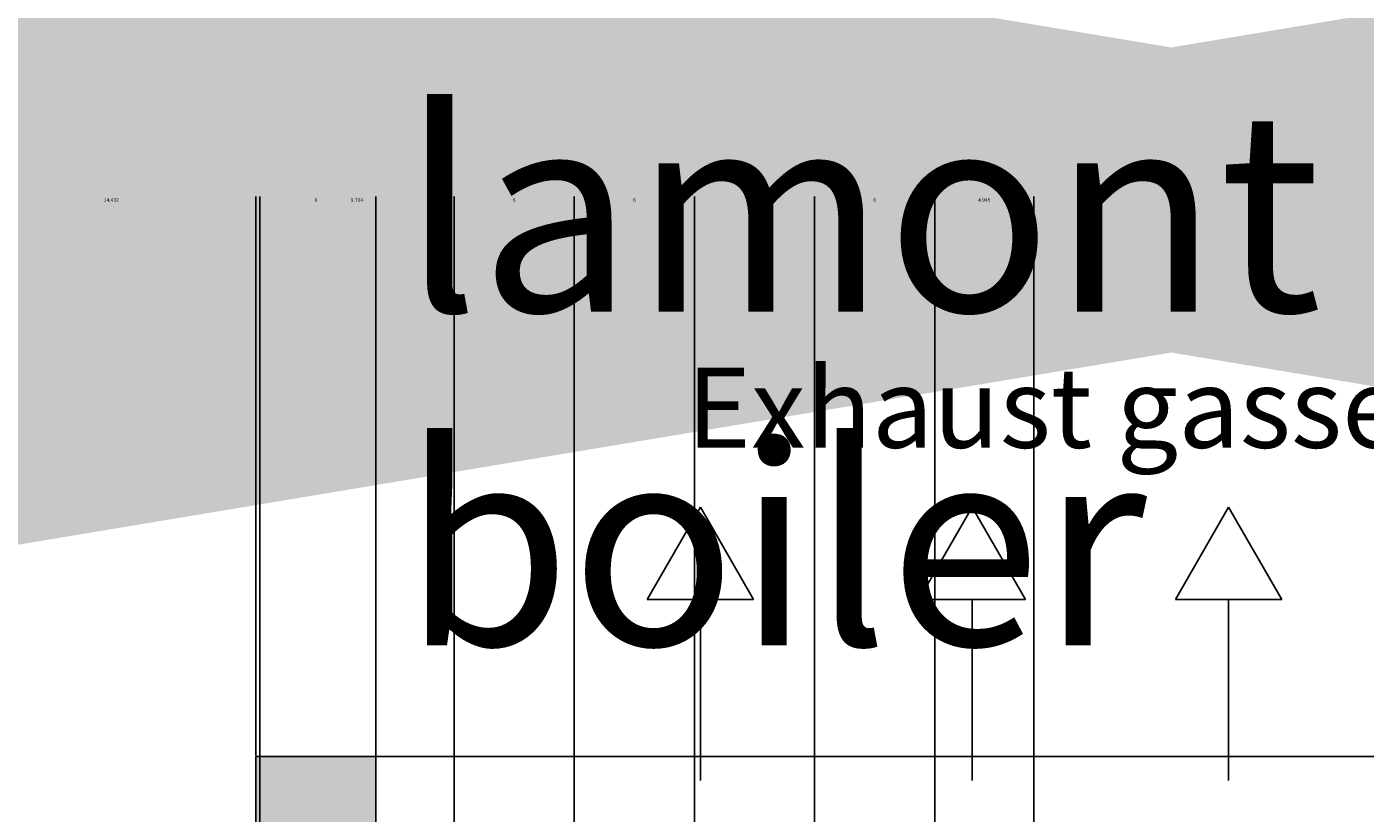
# Model space of a CAD drawing. Units: millimetres. Extents: x -22994 to 29398, y -19990 to 20176.
# Tile 110 of 135: x 99 to 166, y 174 to 213. Entities that reach past the tile are written whole.
import ezdxf

# ---------------------------------------------------------------- set-up
doc = ezdxf.new("R2010")
doc.units = ezdxf.units.MM
doc.header["$MEASUREMENT"] = 0
for name, color, linetype, lineweight in [('M-ANNO-SYMB', 7, 'Continuous', 25), ('M-ANNO-TEXT', 7, 'Continuous', 25), ('M-DIMS', 2, 'Continuous', 18), ('M-EQPM', 7, 'Continuous', 25), ('M-EQPM-PATT', 7, 'Continuous', 18)]:
    doc.layers.add(name, color=color, linetype=linetype, lineweight=lineweight)
doc.styles.get("Standard").update_dxf_attribs({"font": 'arial.ttf'})
doc.dimstyles.get("Standard").update_dxf_attribs({"dimtxt": 0.18, "dimasz": 10000, "dimexe": 0.18, "dimexo": 0.0625, "dimgap": 0.09, "dimtad": 0, "dimtih": 1, "dimtoh": 1, "dimdec": 0, "dimzin": 0, "dimdsep": 46, "dimtxsty": 'Standard', "dimcen": 0.09, "dimadec": 0, "dimazin": 0, "dimtfac": 1, "dimtdec": 0, "dimtofl": 0, "dimtmove": 0, "dimatfit": 3, "dimfxl": 1, "dimtolj": 1, "dimtzin": 0, "dimlwd": 30, "dimarcsym": 0})

# ---------------------------------------------------------------- blocks, each defined once
blk = doc.blocks.new('ARROW-FLOW')
for p, q in [((4.609, 5.322), (0, 2.661)), ((4.609, 5.322), (4.609, 0)), ((4.609, 0), (0, 2.661))]:
    blk.add_line(p, q)
blk = doc.blocks.new('*D2')
at = {"layer": 'Defpoints', "color": 0, "transparency": 16777216}
for p in [(6.677, 10.271), (290.852, 10.271), (290.852, -5.079)]:
    blk.add_point(p, dxfattribs=at)
at = {"layer": 'M-DIMS', "color": 0, "lineweight": -2, "transparency": 16777216}
for p, q in [((6.677, 10.209), (6.677, -5.259)), ((290.852, 10.209), (290.852, -5.259))]:
    blk.add_line(p, q, dxfattribs=at)
at = {"layer": 'M-DIMS', "color": 0, "lineweight": 30, "transparency": 16777216}
for p, q in [((-9993.323, -5.079), (-19993.323, -5.079)), ((10290.852, -5.079), (20290.852, -5.079))]:
    blk.add_line(p, q, dxfattribs=at)
at = {"layer": 'M-DIMS', "color": 0, "transparency": 16777216}
for points in [[(-9993.323, 1661.588), (-9993.323, -1671.745), (6.677, -5.079)], [(10290.852, 1661.588), (10290.852, -1671.745), (290.852, -5.079)]]:
    blk.add_solid(points, dxfattribs=at)
at = {"layer": 'M-DIMS', "color": 0, "transparency": 16777216, "insert": (148.765, -5.079), "char_height": 0.18, "attachment_point": 5}
blk.add_mtext('\\A1;284.2', dxfattribs=at)
blk = doc.blocks.new('*D3')
at = {"layer": 'Defpoints', "color": 0, "transparency": 16777216}
for p in [(110.265, 204.165), (110.265, 176.366), (95.833, 127.967)]:
    blk.add_point(p, dxfattribs=at)
at = {"layer": 'M-DIMS', "color": 0, "lineweight": 30, "transparency": 16777216}
for p, q in [((-9904.167, 204.165), (-19904.167, 204.165)), ((10110.265, 204.165), (20110.265, 204.165))]:
    blk.add_line(p, q, dxfattribs=at)
at = {"layer": 'M-DIMS', "color": 0, "lineweight": -2, "transparency": 16777216}
for p, q in [((95.833, 128.03), (95.833, 204.345)), ((110.265, 176.429), (110.265, 204.345))]:
    blk.add_line(p, q, dxfattribs=at)
at = {"layer": 'M-DIMS', "color": 0, "transparency": 16777216}
for points in [[(-9904.167, 1870.832), (-9904.167, -1462.501), (95.833, 204.165)], [(10110.265, 1870.832), (10110.265, -1462.501), (110.265, 204.165)]]:
    blk.add_solid(points, dxfattribs=at)
at = {"layer": 'M-DIMS', "color": 0, "transparency": 16777216, "insert": (103.049, 204.165), "char_height": 0.18, "attachment_point": 5}
blk.add_mtext('\\A1;14.432', dxfattribs=at)
blk = doc.blocks.new('*D4')
at = {"layer": 'Defpoints', "color": 0, "transparency": 16777216}
for p in [(116.265, 204.165), (110.265, 176.366), (116.265, 176.366)]:
    blk.add_point(p, dxfattribs=at)
at = {"layer": 'M-DIMS', "color": 0, "lineweight": 30, "transparency": 16777216}
for p, q in [((-9889.735, 204.165), (-19889.735, 204.165)), ((10116.265, 204.165), (20116.265, 204.165))]:
    blk.add_line(p, q, dxfattribs=at)
at = {"layer": 'M-DIMS', "color": 0, "lineweight": -2, "transparency": 16777216}
for p, q in [((110.265, 176.429), (110.265, 204.345)), ((116.265, 176.429), (116.265, 204.345))]:
    blk.add_line(p, q, dxfattribs=at)
at = {"layer": 'M-DIMS', "color": 0, "transparency": 16777216}
for points in [[(-9889.735, 1870.832), (-9889.735, -1462.501), (110.265, 204.165)], [(10116.265, 1870.832), (10116.265, -1462.501), (116.265, 204.165)]]:
    blk.add_solid(points, dxfattribs=at)
at = {"layer": 'M-DIMS', "color": 0, "transparency": 16777216, "insert": (113.265, 204.165), "char_height": 0.18, "attachment_point": 5}
blk.add_mtext('\\A1;6', dxfattribs=at)
blk = doc.blocks.new('*D5')
at = {"layer": 'Defpoints', "color": 0, "transparency": 16777216}
for p in [(181.265, 204.165), (116.265, 176.366), (181.265, 176.366)]:
    blk.add_point(p, dxfattribs=at)
at = {"layer": 'M-DIMS', "color": 0, "lineweight": 30, "transparency": 16777216}
for p, q in [((-9883.735, 204.165), (-19883.735, 204.165)), ((10181.265, 204.165), (20181.265, 204.165))]:
    blk.add_line(p, q, dxfattribs=at)
at = {"layer": 'M-DIMS', "color": 0, "lineweight": -2, "transparency": 16777216}
for p, q in [((116.265, 176.429), (116.265, 204.345)), ((181.265, 176.429), (181.265, 204.345))]:
    blk.add_line(p, q, dxfattribs=at)
at = {"layer": 'M-DIMS', "color": 0, "transparency": 16777216}
for points in [[(-9883.735, 1870.832), (-9883.735, -1462.501), (116.265, 204.165)], [(10181.265, 1870.832), (10181.265, -1462.501), (181.265, 204.165)]]:
    blk.add_solid(points, dxfattribs=at)
at = {"layer": 'M-DIMS', "color": 0, "transparency": 16777216, "insert": (148.765, 204.165), "char_height": 0.18, "attachment_point": 5}
blk.add_mtext('\\A1;65', dxfattribs=at)
blk = doc.blocks.new('*D6')
at = {"layer": 'Defpoints', "color": 0, "transparency": 16777216}
for p in [(187.265, 204.165), (181.265, 176.366), (187.265, 176.366)]:
    blk.add_point(p, dxfattribs=at)
at = {"layer": 'M-DIMS', "color": 0, "lineweight": 30, "transparency": 16777216}
for p, q in [((-9818.735, 204.165), (-19818.735, 204.165)), ((10187.265, 204.165), (20187.265, 204.165))]:
    blk.add_line(p, q, dxfattribs=at)
at = {"layer": 'M-DIMS', "color": 0, "lineweight": -2, "transparency": 16777216}
for p, q in [((181.265, 176.429), (181.265, 204.345)), ((187.265, 176.429), (187.265, 204.345))]:
    blk.add_line(p, q, dxfattribs=at)
at = {"layer": 'M-DIMS', "color": 0, "transparency": 16777216}
for points in [[(-9818.735, 1870.832), (-9818.735, -1462.501), (181.265, 204.165)], [(10187.265, 1870.832), (10187.265, -1462.501), (187.265, 204.165)]]:
    blk.add_solid(points, dxfattribs=at)
at = {"layer": 'M-DIMS', "color": 0, "transparency": 16777216, "insert": (184.265, 204.165), "char_height": 0.18, "attachment_point": 5}
blk.add_mtext('\\A1;6', dxfattribs=at)
blk = doc.blocks.new('*D7')
at = {"layer": 'Defpoints', "color": 0, "transparency": 16777216}
for p in [(201.697, 204.165), (187.265, 176.366), (201.697, 127.967)]:
    blk.add_point(p, dxfattribs=at)
at = {"layer": 'M-DIMS', "color": 0, "lineweight": 30, "transparency": 16777216}
for p, q in [((-9812.735, 204.165), (-19812.735, 204.165)), ((10201.697, 204.165), (20201.697, 204.165))]:
    blk.add_line(p, q, dxfattribs=at)
at = {"layer": 'M-DIMS', "color": 0, "lineweight": -2, "transparency": 16777216}
for p, q in [((187.265, 176.429), (187.265, 204.345)), ((201.697, 128.03), (201.697, 204.345))]:
    blk.add_line(p, q, dxfattribs=at)
at = {"layer": 'M-DIMS', "color": 0, "transparency": 16777216}
for points in [[(-9812.735, 1870.832), (-9812.735, -1462.501), (187.265, 204.165)], [(10201.697, 1870.832), (10201.697, -1462.501), (201.697, 204.165)]]:
    blk.add_solid(points, dxfattribs=at)
at = {"layer": 'M-DIMS', "color": 0, "transparency": 16777216, "insert": (194.481, 204.165), "char_height": 0.18, "attachment_point": 5}
blk.add_mtext('\\A1;14.432', dxfattribs=at)
blk = doc.blocks.new('*D8')
at = {"layer": 'Defpoints', "color": 0, "transparency": 16777216}
for p in [(227.648, 204.165), (227.648, 146.73), (201.697, 127.967)]:
    blk.add_point(p, dxfattribs=at)
at = {"layer": 'M-DIMS', "color": 0, "lineweight": 30, "transparency": 16777216}
for p, q in [((-9798.303, 204.165), (-19798.303, 204.165)), ((10227.648, 204.165), (20227.648, 204.165))]:
    blk.add_line(p, q, dxfattribs=at)
at = {"layer": 'M-DIMS', "color": 0, "lineweight": -2, "transparency": 16777216}
for p, q in [((201.697, 128.03), (201.697, 204.345)), ((227.648, 146.792), (227.648, 204.345))]:
    blk.add_line(p, q, dxfattribs=at)
at = {"layer": 'M-DIMS', "color": 0, "transparency": 16777216}
for points in [[(-9798.303, 1870.832), (-9798.303, -1462.501), (201.697, 204.165)], [(10227.648, 1870.832), (10227.648, -1462.501), (227.648, 204.165)]]:
    blk.add_solid(points, dxfattribs=at)
at = {"layer": 'M-DIMS', "color": 0, "transparency": 16777216, "insert": (214.673, 204.165), "char_height": 0.18, "attachment_point": 5}
blk.add_mtext('\\A1;25.95', dxfattribs=at)
blk = doc.blocks.new('*D9')
at = {"layer": 'Defpoints', "color": 0, "transparency": 16777216}
for p in [(187.265, 176.366), (306.202, 176.366), (290.852, 10.271)]:
    blk.add_point(p, dxfattribs=at)
at = {"layer": 'M-DIMS', "color": 0, "lineweight": 30, "transparency": 16777216}
for p, q in [((306.202, 10176.366), (306.202, 20176.366)), ((306.202, -9989.729), (306.202, -19989.729))]:
    blk.add_line(p, q, dxfattribs=at)
at = {"layer": 'M-DIMS', "color": 0, "lineweight": -2, "transparency": 16777216}
for p, q in [((187.327, 176.366), (306.382, 176.366)), ((290.915, 10.271), (306.382, 10.271))]:
    blk.add_line(p, q, dxfattribs=at)
at = {"layer": 'M-DIMS', "color": 0, "transparency": 16777216}
for points in [[(-1360.465, 10176.366), (1972.869, 10176.366), (306.202, 176.366)], [(-1360.465, -9989.729), (1972.869, -9989.729), (306.202, 10.271)]]:
    blk.add_solid(points, dxfattribs=at)
at = {"layer": 'M-DIMS', "color": 0, "transparency": 16777216, "insert": (306.202, 93.319), "char_height": 0.18, "attachment_point": 5}
blk.add_mtext('\\A1;166.1', dxfattribs=at)
blk = doc.blocks.new('*D10')
at = {"layer": 'Defpoints', "color": 0, "transparency": 16777216}
for p in [(125.65, 136.071), (133.346, 136.071), (133.346, -5.079)]:
    blk.add_point(p, dxfattribs=at)
at = {"layer": 'M-DIMS', "color": 0, "lineweight": -2, "transparency": 16777216}
for p, q in [((125.65, 136.009), (125.65, -5.259)), ((133.346, 136.009), (133.346, -5.259))]:
    blk.add_line(p, q, dxfattribs=at)
at = {"layer": 'M-DIMS', "color": 0, "lineweight": 30, "transparency": 16777216}
for p, q in [((-9874.35, -5.079), (-19874.35, -5.079)), ((10133.346, -5.079), (20133.346, -5.079))]:
    blk.add_line(p, q, dxfattribs=at)
at = {"layer": 'M-DIMS', "color": 0, "transparency": 16777216}
for points in [[(-9874.35, 1661.588), (-9874.35, -1671.745), (125.65, -5.079)], [(10133.346, 1661.588), (10133.346, -1671.745), (133.346, -5.079)]]:
    blk.add_solid(points, dxfattribs=at)
at = {"layer": 'M-DIMS', "color": 0, "transparency": 16777216, "insert": (129.498, -5.079), "char_height": 0.18, "attachment_point": 5}
blk.add_mtext('\\A1;7.696', dxfattribs=at)
blk = doc.blocks.new('*D11')
at = {"layer": 'Defpoints', "color": 0, "transparency": 16777216}
for p in [(133.346, 136.071), (135.65, 136.071), (135.65, -5.079)]:
    blk.add_point(p, dxfattribs=at)
at = {"layer": 'M-DIMS', "color": 0, "lineweight": -2, "transparency": 16777216}
for p, q in [((133.346, 136.009), (133.346, -5.259)), ((135.65, 136.009), (135.65, -5.259))]:
    blk.add_line(p, q, dxfattribs=at)
at = {"layer": 'M-DIMS', "color": 0, "lineweight": 30, "transparency": 16777216}
for p, q in [((-9866.654, -5.079), (-19866.654, -5.079)), ((10135.65, -5.079), (20135.65, -5.079))]:
    blk.add_line(p, q, dxfattribs=at)
at = {"layer": 'M-DIMS', "color": 0, "transparency": 16777216}
for points in [[(-9866.654, 1661.588), (-9866.654, -1671.745), (133.346, -5.079)], [(10135.65, 1661.588), (10135.65, -1671.745), (135.65, -5.079)]]:
    blk.add_solid(points, dxfattribs=at)
at = {"layer": 'M-DIMS', "color": 0, "transparency": 16777216, "insert": (134.498, -5.079), "char_height": 0.18, "attachment_point": 5}
blk.add_mtext('\\A1;2.304', dxfattribs=at)
blk = doc.blocks.new('*D12')
at = {"layer": 'Defpoints', "color": 0, "transparency": 16777216}
for p in [(135.65, 136.071), (145.65, 136.071), (145.65, -5.079)]:
    blk.add_point(p, dxfattribs=at)
at = {"layer": 'M-DIMS', "color": 0, "lineweight": -2, "transparency": 16777216}
for p, q in [((135.65, 136.009), (135.65, -5.259)), ((145.65, 136.009), (145.65, -5.259))]:
    blk.add_line(p, q, dxfattribs=at)
at = {"layer": 'M-DIMS', "color": 0, "lineweight": 30, "transparency": 16777216}
for p, q in [((-9864.35, -5.079), (-19864.35, -5.079)), ((10145.65, -5.079), (20145.65, -5.079))]:
    blk.add_line(p, q, dxfattribs=at)
at = {"layer": 'M-DIMS', "color": 0, "transparency": 16777216}
for points in [[(-9864.35, 1661.588), (-9864.35, -1671.745), (135.65, -5.079)], [(10145.65, 1661.588), (10145.65, -1671.745), (145.65, -5.079)]]:
    blk.add_solid(points, dxfattribs=at)
at = {"layer": 'M-DIMS', "color": 0, "transparency": 16777216, "insert": (140.65, -5.079), "char_height": 0.18, "attachment_point": 5}
blk.add_mtext('\\A1;10', dxfattribs=at)
blk = doc.blocks.new('*D13')
at = {"layer": 'Defpoints', "color": 0, "transparency": 16777216}
for p in [(145.65, 136.071), (155.65, 136.071), (155.65, -5.079)]:
    blk.add_point(p, dxfattribs=at)
at = {"layer": 'M-DIMS', "color": 0, "lineweight": -2, "transparency": 16777216}
for p, q in [((145.65, 136.009), (145.65, -5.259)), ((155.65, 136.009), (155.65, -5.259))]:
    blk.add_line(p, q, dxfattribs=at)
at = {"layer": 'M-DIMS', "color": 0, "lineweight": 30, "transparency": 16777216}
for p, q in [((-9854.35, -5.079), (-19854.35, -5.079)), ((10155.65, -5.079), (20155.65, -5.079))]:
    blk.add_line(p, q, dxfattribs=at)
at = {"layer": 'M-DIMS', "color": 0, "transparency": 16777216}
for points in [[(-9854.35, 1661.588), (-9854.35, -1671.745), (145.65, -5.079)], [(10155.65, 1661.588), (10155.65, -1671.745), (155.65, -5.079)]]:
    blk.add_solid(points, dxfattribs=at)
at = {"layer": 'M-DIMS', "color": 0, "transparency": 16777216, "insert": (150.65, -5.079), "char_height": 0.18, "attachment_point": 5}
blk.add_mtext('\\A1;10', dxfattribs=at)
blk = doc.blocks.new('*D14')
at = {"layer": 'Defpoints', "color": 0, "transparency": 16777216}
for p in [(155.65, 136.071), (165.65, 136.071), (165.65, -5.079)]:
    blk.add_point(p, dxfattribs=at)
at = {"layer": 'M-DIMS', "color": 0, "lineweight": -2, "transparency": 16777216}
for p, q in [((155.65, 136.009), (155.65, -5.259)), ((165.65, 136.009), (165.65, -5.259))]:
    blk.add_line(p, q, dxfattribs=at)
at = {"layer": 'M-DIMS', "color": 0, "lineweight": 30, "transparency": 16777216}
for p, q in [((-9844.35, -5.079), (-19844.35, -5.079)), ((10165.65, -5.079), (20165.65, -5.079))]:
    blk.add_line(p, q, dxfattribs=at)
at = {"layer": 'M-DIMS', "color": 0, "transparency": 16777216}
for points in [[(-9844.35, 1661.588), (-9844.35, -1671.745), (155.65, -5.079)], [(10165.65, 1661.588), (10165.65, -1671.745), (165.65, -5.079)]]:
    blk.add_solid(points, dxfattribs=at)
at = {"layer": 'M-DIMS', "color": 0, "transparency": 16777216, "insert": (160.65, -5.079), "char_height": 0.18, "attachment_point": 5}
blk.add_mtext('\\A1;10', dxfattribs=at)
blk = doc.blocks.new('*D15')
at = {"layer": 'Defpoints', "color": 0, "transparency": 16777216}
for p in [(173.346, 154.788), (173.346, 136.071), (306.202, 136.071)]:
    blk.add_point(p, dxfattribs=at)
at = {"layer": 'M-DIMS', "color": 0, "lineweight": 30, "transparency": 16777216}
for p, q in [((306.202, 10154.788), (306.202, 20154.788)), ((306.202, -9863.929), (306.202, -19863.929))]:
    blk.add_line(p, q, dxfattribs=at)
at = {"layer": 'M-DIMS', "color": 0, "lineweight": -2, "transparency": 16777216}
for p, q in [((173.408, 154.788), (306.382, 154.788)), ((173.408, 136.071), (306.382, 136.071))]:
    blk.add_line(p, q, dxfattribs=at)
at = {"layer": 'M-DIMS', "color": 0, "transparency": 16777216}
for points in [[(-1360.465, 10154.788), (1972.869, 10154.788), (306.202, 154.788)], [(-1360.465, -9863.929), (1972.869, -9863.929), (306.202, 136.071)]]:
    blk.add_solid(points, dxfattribs=at)
at = {"layer": 'M-DIMS', "color": 0, "transparency": 16777216, "insert": (306.202, 145.43), "char_height": 0.18, "attachment_point": 5}
blk.add_mtext('\\A1;18.717', dxfattribs=at)
blk = doc.blocks.new('*D16')
at = {"layer": 'Defpoints', "color": 0, "transparency": 16777216}
for p in [(120.17, 204.165), (110.466, 48.035), (120.17, 48.035)]:
    blk.add_point(p, dxfattribs=at)
at = {"layer": 'M-DIMS', "color": 0, "lineweight": 30, "transparency": 16777216}
for p, q in [((-9889.534, 204.165), (-19889.534, 204.165)), ((10120.17, 204.165), (20120.17, 204.165))]:
    blk.add_line(p, q, dxfattribs=at)
at = {"layer": 'M-DIMS', "color": 0, "lineweight": -2, "transparency": 16777216}
for p, q in [((110.466, 48.097), (110.466, 204.345)), ((120.17, 48.097), (120.17, 204.345))]:
    blk.add_line(p, q, dxfattribs=at)
at = {"layer": 'M-DIMS', "color": 0, "transparency": 16777216}
for points in [[(-9889.534, 1870.832), (-9889.534, -1462.501), (110.466, 204.165)], [(10120.17, 1870.832), (10120.17, -1462.501), (120.17, 204.165)]]:
    blk.add_solid(points, dxfattribs=at)
at = {"layer": 'M-DIMS', "color": 0, "transparency": 16777216, "insert": (115.318, 204.165), "char_height": 0.18, "attachment_point": 5}
blk.add_mtext('\\A1;9.704', dxfattribs=at)
blk = doc.blocks.new('*D17')
at = {"layer": 'Defpoints', "color": 0, "transparency": 16777216}
for p in [(126.17, 204.165), (120.17, 48.035), (126.17, 48.035)]:
    blk.add_point(p, dxfattribs=at)
at = {"layer": 'M-DIMS', "color": 0, "lineweight": 30, "transparency": 16777216}
for p, q in [((-9879.83, 204.165), (-19879.83, 204.165)), ((10126.17, 204.165), (20126.17, 204.165))]:
    blk.add_line(p, q, dxfattribs=at)
at = {"layer": 'M-DIMS', "color": 0, "lineweight": -2, "transparency": 16777216}
for p, q in [((120.17, 48.097), (120.17, 204.345)), ((126.17, 48.097), (126.17, 204.345))]:
    blk.add_line(p, q, dxfattribs=at)
at = {"layer": 'M-DIMS', "color": 0, "transparency": 16777216}
for points in [[(-9879.83, 1870.832), (-9879.83, -1462.501), (120.17, 204.165)], [(10126.17, 1870.832), (10126.17, -1462.501), (126.17, 204.165)]]:
    blk.add_solid(points, dxfattribs=at)
at = {"layer": 'M-DIMS', "color": 0, "transparency": 16777216, "insert": (123.17, 204.165), "char_height": 0.18, "attachment_point": 5}
blk.add_mtext('\\A1;6', dxfattribs=at)
blk = doc.blocks.new('*D18')
at = {"layer": 'Defpoints', "color": 0, "transparency": 16777216}
for p in [(132.17, 204.165), (126.17, 48.035), (132.17, 48.035)]:
    blk.add_point(p, dxfattribs=at)
at = {"layer": 'M-DIMS', "color": 0, "lineweight": 30, "transparency": 16777216}
for p, q in [((-9873.83, 204.165), (-19873.83, 204.165)), ((10132.17, 204.165), (20132.17, 204.165))]:
    blk.add_line(p, q, dxfattribs=at)
at = {"layer": 'M-DIMS', "color": 0, "lineweight": -2, "transparency": 16777216}
for p, q in [((126.17, 48.097), (126.17, 204.345)), ((132.17, 48.097), (132.17, 204.345))]:
    blk.add_line(p, q, dxfattribs=at)
at = {"layer": 'M-DIMS', "color": 0, "transparency": 16777216}
for points in [[(-9873.83, 1870.832), (-9873.83, -1462.501), (126.17, 204.165)], [(10132.17, 1870.832), (10132.17, -1462.501), (132.17, 204.165)]]:
    blk.add_solid(points, dxfattribs=at)
at = {"layer": 'M-DIMS', "color": 0, "transparency": 16777216, "insert": (129.17, 204.165), "char_height": 0.18, "attachment_point": 5}
blk.add_mtext('\\A1;6', dxfattribs=at)
blk = doc.blocks.new('*D19')
at = {"layer": 'Defpoints', "color": 0, "transparency": 16777216}
for p in [(138.17, 204.165), (132.17, 48.035), (138.17, 48.035)]:
    blk.add_point(p, dxfattribs=at)
at = {"layer": 'M-DIMS', "color": 0, "lineweight": 30, "transparency": 16777216}
for p, q in [((-9867.83, 204.165), (-19867.83, 204.165)), ((10138.17, 204.165), (20138.17, 204.165))]:
    blk.add_line(p, q, dxfattribs=at)
at = {"layer": 'M-DIMS', "color": 0, "lineweight": -2, "transparency": 16777216}
for p, q in [((132.17, 48.097), (132.17, 204.345)), ((138.17, 48.097), (138.17, 204.345))]:
    blk.add_line(p, q, dxfattribs=at)
at = {"layer": 'M-DIMS', "color": 0, "transparency": 16777216}
for points in [[(-9867.83, 1870.832), (-9867.83, -1462.501), (132.17, 204.165)], [(10138.17, 1870.832), (10138.17, -1462.501), (138.17, 204.165)]]:
    blk.add_solid(points, dxfattribs=at)
at = {"layer": 'M-DIMS', "color": 0, "transparency": 16777216, "insert": (135.17, 204.165), "char_height": 0.18, "attachment_point": 5}
blk.add_mtext('\\A1;6', dxfattribs=at)
blk = doc.blocks.new('*D20')
at = {"layer": 'Defpoints', "color": 0, "transparency": 16777216}
for p in [(144.17, 204.165), (138.17, 48.035), (144.17, 48.035)]:
    blk.add_point(p, dxfattribs=at)
at = {"layer": 'M-DIMS', "color": 0, "lineweight": 30, "transparency": 16777216}
for p, q in [((-9861.83, 204.165), (-19861.83, 204.165)), ((10144.17, 204.165), (20144.17, 204.165))]:
    blk.add_line(p, q, dxfattribs=at)
at = {"layer": 'M-DIMS', "color": 0, "lineweight": -2, "transparency": 16777216}
for p, q in [((138.17, 48.097), (138.17, 204.345)), ((144.17, 48.097), (144.17, 204.345))]:
    blk.add_line(p, q, dxfattribs=at)
at = {"layer": 'M-DIMS', "color": 0, "transparency": 16777216}
for points in [[(-9861.83, 1870.832), (-9861.83, -1462.501), (138.17, 204.165)], [(10144.17, 1870.832), (10144.17, -1462.501), (144.17, 204.165)]]:
    blk.add_solid(points, dxfattribs=at)
at = {"layer": 'M-DIMS', "color": 0, "transparency": 16777216, "insert": (141.17, 204.165), "char_height": 0.18, "attachment_point": 5}
blk.add_mtext('\\A1;6', dxfattribs=at)
blk = doc.blocks.new('*D21')
at = {"layer": 'Defpoints', "color": 0, "transparency": 16777216}
for p in [(149.116, 204.165), (144.17, 48.035), (149.116, 48.035)]:
    blk.add_point(p, dxfattribs=at)
at = {"layer": 'M-DIMS', "color": 0, "lineweight": 30, "transparency": 16777216}
for p, q in [((-9855.83, 204.165), (-19855.83, 204.165)), ((10149.116, 204.165), (20149.116, 204.165))]:
    blk.add_line(p, q, dxfattribs=at)
at = {"layer": 'M-DIMS', "color": 0, "lineweight": -2, "transparency": 16777216}
for p, q in [((144.17, 48.097), (144.17, 204.345)), ((149.116, 48.097), (149.116, 204.345))]:
    blk.add_line(p, q, dxfattribs=at)
at = {"layer": 'M-DIMS', "color": 0, "transparency": 16777216}
for points in [[(-9855.83, 1870.832), (-9855.83, -1462.501), (144.17, 204.165)], [(10149.116, 1870.832), (10149.116, -1462.501), (149.116, 204.165)]]:
    blk.add_solid(points, dxfattribs=at)
at = {"layer": 'M-DIMS', "color": 0, "transparency": 16777216, "insert": (146.643, 204.165), "char_height": 0.18, "attachment_point": 5}
blk.add_mtext('\\A1;4.945', dxfattribs=at)
blk = doc.blocks.new('*D22')
at = {"layer": 'Defpoints', "color": 0, "transparency": 16777216}
for p in [(149.116, 30.99), (155.116, 30.99), (155.116, -5.079)]:
    blk.add_point(p, dxfattribs=at)
at = {"layer": 'M-DIMS', "color": 0, "lineweight": -2, "transparency": 16777216}
for p, q in [((149.116, 30.927), (149.116, -5.259)), ((155.116, 30.927), (155.116, -5.259))]:
    blk.add_line(p, q, dxfattribs=at)
at = {"layer": 'M-DIMS', "color": 0, "lineweight": 30, "transparency": 16777216}
for p, q in [((-9850.884, -5.079), (-19850.884, -5.079)), ((10155.116, -5.079), (20155.116, -5.079))]:
    blk.add_line(p, q, dxfattribs=at)
at = {"layer": 'M-DIMS', "color": 0, "transparency": 16777216}
for points in [[(-9850.884, 1661.588), (-9850.884, -1671.745), (149.116, -5.079)], [(10155.116, 1661.588), (10155.116, -1671.745), (155.116, -5.079)]]:
    blk.add_solid(points, dxfattribs=at)
at = {"layer": 'M-DIMS', "color": 0, "transparency": 16777216, "insert": (152.116, -5.079), "char_height": 0.18, "attachment_point": 5}
blk.add_mtext('\\A1;6', dxfattribs=at)
blk = doc.blocks.new('*D23')
at = {"layer": 'Defpoints', "color": 0, "transparency": 16777216}
for p in [(155.116, 30.99), (161.116, 30.99), (161.116, -5.079)]:
    blk.add_point(p, dxfattribs=at)
at = {"layer": 'M-DIMS', "color": 0, "lineweight": -2, "transparency": 16777216}
for p, q in [((155.116, 30.927), (155.116, -5.259)), ((161.116, 30.927), (161.116, -5.259))]:
    blk.add_line(p, q, dxfattribs=at)
at = {"layer": 'M-DIMS', "color": 0, "lineweight": 30, "transparency": 16777216}
for p, q in [((-9844.884, -5.079), (-19844.884, -5.079)), ((10161.116, -5.079), (20161.116, -5.079))]:
    blk.add_line(p, q, dxfattribs=at)
at = {"layer": 'M-DIMS', "color": 0, "transparency": 16777216}
for points in [[(-9844.884, 1661.588), (-9844.884, -1671.745), (155.116, -5.079)], [(10161.116, 1661.588), (10161.116, -1671.745), (161.116, -5.079)]]:
    blk.add_solid(points, dxfattribs=at)
at = {"layer": 'M-DIMS', "color": 0, "transparency": 16777216, "insert": (158.116, -5.079), "char_height": 0.18, "attachment_point": 5}
blk.add_mtext('\\A1;6', dxfattribs=at)
blk = doc.blocks.new('*D24')
at = {"layer": 'Defpoints', "color": 0, "transparency": 16777216}
for p in [(161.116, 30.99), (166.439, 30.99), (166.439, -5.079)]:
    blk.add_point(p, dxfattribs=at)
at = {"layer": 'M-DIMS', "color": 0, "lineweight": -2, "transparency": 16777216}
for p, q in [((161.116, 30.927), (161.116, -5.259)), ((166.439, 30.927), (166.439, -5.259))]:
    blk.add_line(p, q, dxfattribs=at)
at = {"layer": 'M-DIMS', "color": 0, "lineweight": 30, "transparency": 16777216}
for p, q in [((-9838.884, -5.079), (-19838.884, -5.079)), ((10166.439, -5.079), (20166.439, -5.079))]:
    blk.add_line(p, q, dxfattribs=at)
at = {"layer": 'M-DIMS', "color": 0, "transparency": 16777216}
for points in [[(-9838.884, 1661.588), (-9838.884, -1671.745), (161.116, -5.079)], [(10166.439, 1661.588), (10166.439, -1671.745), (166.439, -5.079)]]:
    blk.add_solid(points, dxfattribs=at)
at = {"layer": 'M-DIMS', "color": 0, "transparency": 16777216, "insert": (163.777, -5.079), "char_height": 0.18, "attachment_point": 5}
blk.add_mtext('\\A1;5.323', dxfattribs=at)
blk = doc.blocks.new('*D25')
at = {"layer": 'Defpoints', "color": 0, "transparency": 16777216}
for p in [(166.439, 30.99), (172.439, 30.99), (172.439, -5.079)]:
    blk.add_point(p, dxfattribs=at)
at = {"layer": 'M-DIMS', "color": 0, "lineweight": -2, "transparency": 16777216}
for p, q in [((166.439, 30.927), (166.439, -5.259)), ((172.439, 30.927), (172.439, -5.259))]:
    blk.add_line(p, q, dxfattribs=at)
at = {"layer": 'M-DIMS', "color": 0, "lineweight": 30, "transparency": 16777216}
for p, q in [((-9833.561, -5.079), (-19833.561, -5.079)), ((10172.439, -5.079), (20172.439, -5.079))]:
    blk.add_line(p, q, dxfattribs=at)
at = {"layer": 'M-DIMS', "color": 0, "transparency": 16777216}
for points in [[(-9833.561, 1661.588), (-9833.561, -1671.745), (166.439, -5.079)], [(10172.439, 1661.588), (10172.439, -1671.745), (172.439, -5.079)]]:
    blk.add_solid(points, dxfattribs=at)
at = {"layer": 'M-DIMS', "color": 0, "transparency": 16777216, "insert": (169.439, -5.079), "char_height": 0.18, "attachment_point": 5}
blk.add_mtext('\\A1;6', dxfattribs=at)
blk = doc.blocks.new('*D26')
at = {"layer": 'Defpoints', "color": 0, "transparency": 16777216}
for p in [(172.439, 30.99), (178.439, 30.99), (178.439, -5.079)]:
    blk.add_point(p, dxfattribs=at)
at = {"layer": 'M-DIMS', "color": 0, "lineweight": -2, "transparency": 16777216}
for p, q in [((172.439, 30.927), (172.439, -5.259)), ((178.439, 30.927), (178.439, -5.259))]:
    blk.add_line(p, q, dxfattribs=at)
at = {"layer": 'M-DIMS', "color": 0, "lineweight": 30, "transparency": 16777216}
for p, q in [((-9827.561, -5.079), (-19827.561, -5.079)), ((10178.439, -5.079), (20178.439, -5.079))]:
    blk.add_line(p, q, dxfattribs=at)
at = {"layer": 'M-DIMS', "color": 0, "transparency": 16777216}
for points in [[(-9827.561, 1661.588), (-9827.561, -1671.745), (172.439, -5.079)], [(10178.439, 1661.588), (10178.439, -1671.745), (178.439, -5.079)]]:
    blk.add_solid(points, dxfattribs=at)
at = {"layer": 'M-DIMS', "color": 0, "transparency": 16777216, "insert": (175.439, -5.079), "char_height": 0.18, "attachment_point": 5}
blk.add_mtext('\\A1;6', dxfattribs=at)
blk = doc.blocks.new('*D27')
at = {"layer": 'Defpoints', "color": 0, "transparency": 16777216}
for p in [(178.439, 30.99), (188.117, 30.99), (188.117, -5.079)]:
    blk.add_point(p, dxfattribs=at)
at = {"layer": 'M-DIMS', "color": 0, "lineweight": -2, "transparency": 16777216}
for p, q in [((178.439, 30.927), (178.439, -5.259)), ((188.117, 30.927), (188.117, -5.259))]:
    blk.add_line(p, q, dxfattribs=at)
at = {"layer": 'M-DIMS', "color": 0, "lineweight": 30, "transparency": 16777216}
for p, q in [((-9821.561, -5.079), (-19821.561, -5.079)), ((10188.117, -5.079), (20188.117, -5.079))]:
    blk.add_line(p, q, dxfattribs=at)
at = {"layer": 'M-DIMS', "color": 0, "transparency": 16777216}
for points in [[(-9821.561, 1661.588), (-9821.561, -1671.745), (178.439, -5.079)], [(10188.117, 1661.588), (10188.117, -1671.745), (188.117, -5.079)]]:
    blk.add_solid(points, dxfattribs=at)
at = {"layer": 'M-DIMS', "color": 0, "transparency": 16777216, "insert": (183.278, -5.079), "char_height": 0.18, "attachment_point": 5}
blk.add_mtext('\\A1;9.679', dxfattribs=at)
blk = doc.blocks.new('*D28')
at = {"layer": 'Defpoints', "color": 0, "transparency": 16777216}
for p in [(188.117, 48.035), (306.202, 48.035), (188.117, 30.99)]:
    blk.add_point(p, dxfattribs=at)
at = {"layer": 'M-DIMS', "color": 0, "lineweight": 30, "transparency": 16777216}
for p, q in [((306.202, 10048.035), (306.202, 20048.035)), ((306.202, -9969.01), (306.202, -19969.01))]:
    blk.add_line(p, q, dxfattribs=at)
at = {"layer": 'M-DIMS', "color": 0, "lineweight": -2, "transparency": 16777216}
for p, q in [((188.18, 48.035), (306.382, 48.035)), ((188.18, 30.99), (306.382, 30.99))]:
    blk.add_line(p, q, dxfattribs=at)
at = {"layer": 'M-DIMS', "color": 0, "transparency": 16777216}
for points in [[(-1360.465, 10048.035), (1972.869, 10048.035), (306.202, 48.035)], [(-1360.465, -9969.01), (1972.869, -9969.01), (306.202, 30.99)]]:
    blk.add_solid(points, dxfattribs=at)
at = {"layer": 'M-DIMS', "color": 0, "transparency": 16777216, "insert": (306.202, 39.512), "char_height": 0.18, "attachment_point": 5}
blk.add_mtext('\\A1;17.045', dxfattribs=at)
blk = doc.blocks.new('*D29')
at = {"layer": 'Defpoints', "color": 0, "transparency": 16777216}
for p in [(36.801, 80.045), (64.03, 80.045)]:
    blk.add_point(p, dxfattribs=at)
at = {"layer": 'M-DIMS', "color": 0, "lineweight": -2, "transparency": 16777216}
for p, q in [((50.325, 80.045), (50.505, 80.045)), ((50.415, 79.955), (50.415, 80.135))]:
    blk.add_line(p, q, dxfattribs=at)
at = {"layer": 'M-DIMS', "color": 0, "lineweight": 30, "transparency": 16777216}
blk.add_line((20064.03, 80.03), (10064.03, 80.038), dxfattribs=at)
at = {"layer": 'M-DIMS', "color": 0, "transparency": 16777216}
blk.add_solid([(10064.031, 1746.704), (10064.028, -1586.629), (64.03, 80.045)], dxfattribs=at)
at = {"layer": 'M-DIMS', "color": 0, "transparency": 16777216, "insert": (20064.521, 80.03), "char_height": 0.18, "attachment_point": 5}
blk.add_mtext('\\A1;∅27.23', dxfattribs=at)
blk = doc.blocks.new('*D36')
at = {"layer": 'Defpoints', "color": 0, "transparency": 16777216}
for p in [(46.39, 31.303), (46.387, 26.593)]:
    blk.add_point(p, dxfattribs=at)
at = {"layer": 'M-DIMS', "color": 0, "lineweight": 30, "transparency": 16777216}
for p, q in [((57.15, 20031.301), (51.77, 10031.302)), ((10057.15, 20031.301), (57.15, 20031.301))]:
    blk.add_line(p, q, dxfattribs=at)
at = {"layer": 'M-DIMS', "color": 0, "lineweight": -2, "transparency": 16777216}
for p, q in [((46.299, 28.948), (46.479, 28.948)), ((46.389, 28.858), (46.389, 29.038))]:
    blk.add_line(p, q, dxfattribs=at)
at = {"layer": 'M-DIMS', "color": 0, "transparency": 16777216}
blk.add_solid([(-1614.896, 10032.199), (1718.436, 10030.405), (46.39, 31.303)], dxfattribs=at)
at = {"layer": 'M-DIMS', "color": 0, "transparency": 16777216, "insert": (10057.554, 20031.301), "char_height": 0.18, "attachment_point": 5}
blk.add_mtext('\\A1;∅4.71', dxfattribs=at)
blk = doc.blocks.new('*D37')
at = {"layer": 'Defpoints', "color": 0, "transparency": 16777216}
for p in [(54.834, 118.615), (59.494, 118.614)]:
    blk.add_point(p, dxfattribs=at)
at = {"layer": 'M-DIMS', "color": 0, "lineweight": -2, "transparency": 16777216}
for p, q in [((57.074, 118.614), (57.254, 118.614)), ((57.164, 118.524), (57.164, 118.704))]:
    blk.add_line(p, q, dxfattribs=at)
at = {"layer": 'M-DIMS', "color": 0, "lineweight": 30, "transparency": 16777216}
blk.add_line((20059.493, 116.253), (10059.494, 117.434), dxfattribs=at)
at = {"layer": 'M-DIMS', "color": 0, "transparency": 16777216}
blk.add_solid([(10059.69, 1784.1), (10059.297, -1549.233), (59.494, 118.614)], dxfattribs=at)
at = {"layer": 'M-DIMS', "color": 0, "transparency": 16777216, "insert": (20059.985, 116.253), "char_height": 0.18, "attachment_point": 5}
blk.add_mtext('\\A1;∅4.659', dxfattribs=at)

msp = doc.modelspace()

# ---------------------------------------------------------------- hatches: boundary and pattern name
at = {"layer": 'M-EQPM-PATT'}
h = msp.add_hatch(color=256, dxfattribs=at)
h.set_gradient(color1=(205, 32, 39), color2=(205, 32, 39), tint=1)
h.paths.add_polyline_path([(116.2647, 150.3662), (116.2647, 170.3662), (116.2647, 176.3662), (110.2647, 176.3662), (110.2647, 152.0276), (95.8327, 127.967), (95.8327, 16.6063), (201.6967, 16.6063), (201.6967, 127.967), (187.2647, 152.0276), (187.2647, 176.3662), (181.2647, 176.3662), (181.2647, 170.3662), (181.2647, 150.3662), (195.6967, 126.3055), (195.6967, 22.6063), (101.8327, 22.6063), (101.8327, 126.3055)])
h.paths.add_polyline_path([(185.2208, 88.6347), (101.8327, 88.6347), (101.8327, 87.6347), (182.8066, 87.6347), (178.7313, 83.5594), (195.6967, 83.5594), (195.6967, 84.5594), (181.1455, 84.5594)], flags=17)
h.paths.add_polyline_path([(95.8327, 88.6347), (60.9779, 88.6347, -0.0228552), (61.7178, 87.6347), (95.8327, 87.6347)])
h.paths.add_polyline_path([(215.6212, 86.5189), (215.6212, 80.5999), (220.5095, 83.5594)])
h.paths.add_polyline_path([(215.6212, 84.5594), (201.6967, 84.5594), (201.6967, 83.5594), (215.6212, 83.5594)])
h.paths.add_polyline_path([(225.3978, 86.5189), (220.5095, 83.5594), (225.3978, 80.5999)])
h.paths.add_polyline_path([(231.6256, 84.5594), (225.3978, 84.5594), (225.3978, 83.5594), (231.6256, 83.5594)])

# ---------------------------------------------------------------- linework, layer by layer
at = {"layer": 'M-ANNO-SYMB'}
for p, q in [((132.4652, 184.2067), (132.4652, 175.1778)), ((146.0428, 184.2067), (146.0428, 175.1778)), ((158.8445, 184.2067), (158.8445, 175.1778))]:
    msp.add_line(p, q, dxfattribs=at)
at = {"layer": 'M-EQPM'}
msp.add_line((116.2647, 170.3662), (116.2647, 176.3662), dxfattribs=at)
msp.add_lwpolyline([(110.2647, 176.3662), (110.2647, 152.0276), (95.8327, 127.967), (95.8327, 16.6063), (201.6967, 16.6063), (201.6967, 127.967), (187.2647, 152.0276), (187.2647, 176.3662)], close=True, dxfattribs=at)

# ---------------------------------------------------------------- block references
at = {"layer": 'M-ANNO-SYMB', "rotation": 29.99999999999952}
for p in [(131.1348, 181.9021), (144.7123, 181.9021), (157.514, 181.9021)]:
    msp.add_blockref('ARROW-FLOW', p, dxfattribs=at)

# ---------------------------------------------------------------- texts
at = {"layer": 'M-ANNO-TEXT', "attachment_point": 1}
for s, width, insert, char_height in [('lamont boiler', 82.985137, (117.5663, 208.5925), 10), ('Exhaust gasses', 53.370884, (131.7841, 195.7877), 4)]:
    msp.add_mtext_dynamic_manual_height_columns(s, width=width, gutter_width=1, heights=[0], dxfattribs=dict(at, insert=insert, char_height=char_height))

# ---------------------------------------------------------------- dimensions: what is measured, and where the dimension line sits
at = {"layer": 'M-DIMS'}
for base, p1, p2, override, picture, middle in [((306.202, 176.3662), (290.852, 10.2713), (187.2647, 176.3662), {"dimdec": 1, "dimlfac": 1, "dimrnd": 0, "dimzin": 0, "dimdsep": 46, "dimlunit": 2}, '*D9', (306.202, 93.3187)), ((306.202, 136.0713), (173.3459, 154.788), (173.3459, 136.0713), {"dimdec": 3, "dimlfac": 1, "dimrnd": 0, "dimzin": 0, "dimdsep": 46, "dimlunit": 2}, '*D15', (306.202, 145.4297)), ((306.202, 48.0349), (188.1175, 30.9895), (188.1175, 48.0349), {"dimdec": 3, "dimlfac": 1, "dimrnd": 0, "dimzin": 0, "dimdsep": 46, "dimlunit": 2}, '*D28', (306.202, 39.5122))]:
    dim = msp.add_linear_dim(base=base, p1=p1, p2=p2, angle=90, dimstyle='Standard', override=override, dxfattribs=at)
    dim.commit()
    dim.dimension.update_dxf_attribs({"geometry": picture, "text_midpoint": middle})
dim = msp.add_diameter_dim_2p(p1=(46.3875, 26.5934), p2=(46.39, 31.3035), dimstyle='Standard', override={"dimdec": 2, "dimlfac": 1, "dimrnd": 0, "dimzin": 0, "dimdsep": 46, "dimlunit": 2}, dxfattribs=at)
dim.commit()
dim.dimension.update_dxf_attribs({"geometry": '*D36', "text_midpoint": (10057.5542, 20031.3006), "dimtype": 163})
for base, p1, p2, override, picture, middle in [((110.2647, 204.1654), (95.8327, 127.967), (110.2647, 176.3662), {"dimdec": 3, "dimlfac": 1, "dimrnd": 0, "dimzin": 0, "dimdsep": 46, "dimlunit": 2}, '*D3', (103.0487, 204.1654)), ((116.2647, 204.1654), (110.2647, 176.3662), (116.2647, 176.3662), {"dimdec": 0, "dimlfac": 1, "dimrnd": 0, "dimzin": 0, "dimdsep": 46, "dimlunit": 2}, '*D4', (113.2647, 204.1654)), ((120.1702, 204.1654), (110.4658, 48.0349), (120.1702, 48.0349), {"dimdec": 3, "dimlfac": 1, "dimrnd": 0, "dimzin": 0, "dimdsep": 46, "dimlunit": 2}, '*D16', (115.318, 204.1654)), ((181.2647, 204.1654), (116.2647, 176.3662), (181.2647, 176.3662), {"dimdec": 0, "dimlfac": 1, "dimrnd": 0, "dimzin": 0, "dimdsep": 46, "dimlunit": 2}, '*D5', (148.7647, 204.1654)), ((126.1702, 204.1654), (120.1702, 48.0349), (126.1702, 48.0349), {"dimdec": 0, "dimlfac": 1, "dimrnd": 0, "dimzin": 0, "dimdsep": 46, "dimlunit": 2}, '*D17', (123.1702, 204.1654)), ((132.1702, 204.1654), (126.1702, 48.0349), (132.1702, 48.0349), {"dimdec": 0, "dimlfac": 1, "dimrnd": 0, "dimzin": 0, "dimdsep": 46, "dimlunit": 2}, '*D18', (129.1702, 204.1654)), ((138.1702, 204.1654), (132.1702, 48.0349), (138.1702, 48.0349), {"dimdec": 0, "dimlfac": 1, "dimrnd": 0, "dimzin": 0, "dimdsep": 46, "dimlunit": 2}, '*D19', (135.1702, 204.1654)), ((144.1702, 204.1654), (138.1702, 48.0349), (144.1702, 48.0349), {"dimdec": 0, "dimlfac": 1, "dimrnd": 0, "dimzin": 0, "dimdsep": 46, "dimlunit": 2}, '*D20', (141.1702, 204.1654)), ((149.11567, 204.16539), (144.17023, 48.03494), (149.11567, 48.03494), {"dimdec": 3, "dimlfac": 1, "dimrnd": 0, "dimzin": 0, "dimdsep": 46, "dimlunit": 2}, '*D21', (146.64295, 204.16539)), ((187.2647, 204.1654), (181.2647, 176.3662), (187.2647, 176.3662), {"dimdec": 0, "dimlfac": 1, "dimrnd": 0, "dimzin": 0, "dimdsep": 46, "dimlunit": 2}, '*D6', (184.2647, 204.1654)), ((201.6967, 204.1654), (187.2647, 176.3662), (201.6967, 127.967), {"dimdec": 3, "dimlfac": 1, "dimrnd": 0, "dimzin": 0, "dimdsep": 46, "dimlunit": 2}, '*D7', (194.4807, 204.1654)), ((227.6485, 204.1654), (201.6967, 127.967), (227.6485, 146.7296), {"dimdec": 2, "dimlfac": 1, "dimrnd": 0, "dimzin": 0, "dimdsep": 46, "dimlunit": 2}, '*D8', (214.6726, 204.1654)), ((290.852, -5.0787), (6.6773, 10.2713), (290.852, 10.2713), {"dimdec": 1, "dimlfac": 1, "dimrnd": 0, "dimzin": 0, "dimdsep": 46, "dimlunit": 2}, '*D2', (148.7647, -5.0787)), ((133.3459, -5.0787), (125.6498, 136.0713), (133.3459, 136.0713), {"dimdec": 3, "dimlfac": 1, "dimrnd": 0, "dimzin": 0, "dimdsep": 46, "dimlunit": 2}, '*D10', (129.4978, -5.0787)), ((135.6498, -5.0787), (133.3459, 136.0713), (135.6498, 136.0713), {"dimdec": 3, "dimlfac": 1, "dimrnd": 0, "dimzin": 0, "dimdsep": 46, "dimlunit": 2}, '*D11', (134.4978, -5.0787)), ((145.6498, -5.0787), (135.6498, 136.0713), (145.6498, 136.0713), {"dimdec": 0, "dimlfac": 1, "dimrnd": 0, "dimzin": 0, "dimdsep": 46, "dimlunit": 2}, '*D12', (140.6498, -5.0787)), ((155.6498, -5.0787), (145.6498, 136.0713), (155.6498, 136.0713), {"dimdec": 0, "dimlfac": 1, "dimrnd": 0, "dimzin": 0, "dimdsep": 46, "dimlunit": 2}, '*D13', (150.6498, -5.0787)), ((155.1157, -5.0787), (149.1157, 30.9895), (155.1157, 30.9895), {"dimdec": 0, "dimlfac": 1, "dimrnd": 0, "dimzin": 0, "dimdsep": 46, "dimlunit": 2}, '*D22', (152.1157, -5.0787)), ((161.1157, -5.0787), (155.1157, 30.9895), (161.1157, 30.9895), {"dimdec": 0, "dimlfac": 1, "dimrnd": 0, "dimzin": 0, "dimdsep": 46, "dimlunit": 2}, '*D23', (158.1157, -5.0787)), ((165.6498, -5.0787), (155.6498, 136.0713), (165.6498, 136.0713), {"dimdec": 0, "dimlfac": 1, "dimrnd": 0, "dimzin": 0, "dimdsep": 46, "dimlunit": 2}, '*D14', (160.6498, -5.0787)), ((166.4387, -5.0787), (161.1157, 30.9895), (166.4387, 30.9895), {"dimdec": 3, "dimlfac": 1, "dimrnd": 0, "dimzin": 0, "dimdsep": 46, "dimlunit": 2}, '*D24', (163.7772, -5.0787)), ((172.4387, -5.0787), (166.4387, 30.9895), (172.4387, 30.9895), {"dimdec": 0, "dimlfac": 1, "dimrnd": 0, "dimzin": 0, "dimdsep": 46, "dimlunit": 2}, '*D25', (169.4387, -5.0787)), ((178.4387, -5.0787), (172.4387, 30.9895), (178.4387, 30.9895), {"dimdec": 0, "dimlfac": 1, "dimrnd": 0, "dimzin": 0, "dimdsep": 46, "dimlunit": 2}, '*D26', (175.4387, -5.0787)), ((188.1175, -5.0787), (178.4387, 30.9895), (188.1175, 30.9895), {"dimdec": 3, "dimlfac": 1, "dimrnd": 0, "dimzin": 0, "dimdsep": 46, "dimlunit": 2}, '*D27', (183.2781, -5.0787))]:
    dim = msp.add_linear_dim(base=base, p1=p1, p2=p2, dimstyle='Standard', override=override, dxfattribs=at)
    dim.commit()
    dim.dimension.update_dxf_attribs({"geometry": picture, "text_midpoint": middle})
for p1, p2, override, picture, middle in [((54.8343, 118.6145), (59.4936, 118.614), {"dimdec": 3, "dimlfac": 1, "dimrnd": 0, "dimzin": 0, "dimdsep": 46, "dimlunit": 2}, '*D37', (20059.4934, 116.2531)), ((36.8006, 80.045), (64.0296, 80.045), {"dimdec": 2, "dimlfac": 1, "dimrnd": 0, "dimzin": 0, "dimdsep": 46, "dimlunit": 2}, '*D29', (20064.0296, 80.0303))]:
    dim = msp.add_diameter_dim_2p(p1=p1, p2=p2, dimstyle='Standard', override=override, dxfattribs=at)
    dim.commit()
    dim.dimension.update_dxf_attribs({"geometry": picture, "text_midpoint": middle})

doc.saveas('drawing.dxf')
